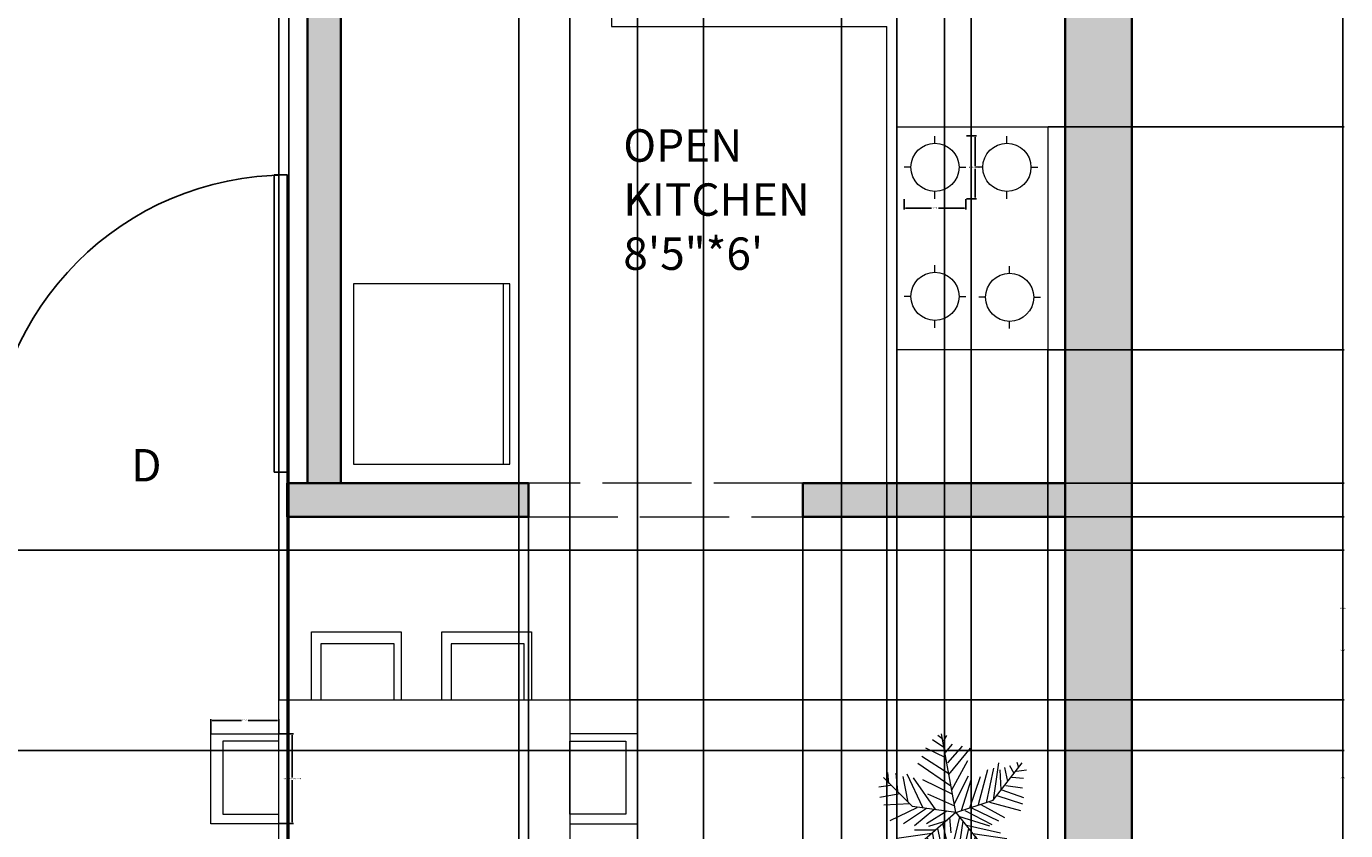
# Model space of a CAD drawing. Units: inches. Extents: x 2035 to 2384, y 1427 to 2020.
# Tile 6 of 7: x 2206 to 2384, y 1794 to 1902. Entities that reach past the tile are written whole.
import ezdxf

# ---------------------------------------------------------------- set-up
doc = ezdxf.new("R2010")
doc.units = ezdxf.units.IN
doc.linetypes.add('ACAD_ISO02W100', pattern=[15, 12, -3])
for name, color, linetype, lineweight in [('A-ANNO-DIMS', 2, 'Continuous', 18), ('A-ANNO-IDEN', 201, 'Continuous', 18), ('A-AREA-IDEN', 201, 'Continuous', 18), ('A-EQPM', 71, 'Continuous', 18), ('A-FLOR-CABN', 71, 'Continuous', 18), ('A-WALL-OVHD', 140, 'ACAD_ISO02W100', 18), ('A-WALL-PATT', 140, 'Continuous', 13), ('C-PROP', 7, 'Continuous', 25), ('DOOR', 52, 'Continuous', 25), ('FUR', 71, 'Continuous', 18), ('L-PLNT', 112, 'Continuous', 18), ('WALL', 140, 'Continuous', 35)]:
    doc.layers.add(name, color=color, linetype=linetype, lineweight=lineweight)
doc.styles.get("Standard").update_dxf_attribs({"font": 'arial.ttf'})
doc.dimstyles.get("Standard").update_dxf_attribs({"dimtxt": 0.18, "dimasz": 0.18, "dimexe": 0.18, "dimexo": 0.0625, "dimgap": 0.09, "dimtad": 0, "dimtih": 1, "dimtoh": 1, "dimdec": 4, "dimzin": 0, "dimdsep": 46, "dimtxsty": 'Standard', "dimcen": 0.09, "dimadec": 0, "dimazin": 0, "dimtfac": 1, "dimtdec": 4, "dimtofl": 0, "dimtmove": 0, "dimatfit": 3, "dimfxl": 1, "dimtolj": 1, "dimtzin": 0, "dimarcsym": 0})

# ---------------------------------------------------------------- blocks, each defined once
blk = doc.blocks.new('*U2')
for p, q in [((0, 0), (0, -6)), ((40, 0), (40, -6))]:
    blk.add_line(p, q)
blk.add_lwpolyline([(0, 0), (0, 40), (1.75, 40), (1.75, 0)], close=True)
blk.add_arc((0, 0), 40, 0, 90)
blk = doc.blocks.new('*U6')
for p, q in [((-8.737, 47.138), (-17.069, 52.711)), ((-10.186, 53.64), (-13.084, 55.962)), ((0, 0), (-10.5, 57)), ((-9.099, 51.782), (-6.563, 55.962)), ((-7.65, 43.423), (-2.578, 49.46)), ((-5.839, 35.992), (4.667, 48.067)), ((-5.114, 28.097), (-24.676, 40.636)), ((-7.288, 39.707), (-21.778, 46.673)), ((-5.114, 27.632), (10.463, 46.673)), ((-48.585, 21.131), (-49.309, 29.026)), ((-3.665, 19.273), (-27.574, 35.527)), ((-2.941, 16.486), (8.652, 37.85)), ((16.259, 5.805), (23.142, 31.348)), ((22.055, 7.198), (27.489, 32.277)), ((27, 9), (48, 36)), ((27.127, 9.056), (31.112, 35.992)), ((31.836, 30.883), (32.561, 16.486)), ((35.096, 32.741), (37.27, 22.524)), ((38.719, 34.134), (41.979, 28.561)), ((43.791, 29.954), (51.036, 30.883)), ((44.153, 36.456), (45.239, 32.741)), ((-47.498, 19.737), (-55.83, 18.344)), ((-31.5, 4.5), (-52.5, 25.5)), ((-43.513, 28.561), (-42.427, 15.558)), ((-38.442, 26.239), (-34.819, 7.663)), ((-35.544, 28.097), (-24.314, 3.947)), ((-14.533, 2.09), (-30.834, 25.31)), ((-24.314, 23.917), (-2.941, 13.7)), ((-1.129, 6.734), (9.014, 26.704)), ((3.942, 1.625), (11.187, 24.381)), ((10.101, 3.483), (17.708, 26.239)), ((36.183, 19.737), (48.137, 17.88)), ((40.53, 25.775), (48.862, 24.846)), ((-40.615, 13.7), (-55.105, 10.913)), ((-20.691, 13.7), (-1.129, 4.876)), ((29.662, 12.307), (48.137, 6.269)), ((33.285, 16.486), (48.862, 10.913)), ((-33.37, 6.269), (-52.207, 5.34)), ((-28.299, 3.483), (-47.86, -5.805)), ((-21.416, 3.018), (-38.079, -8.128)), ((0, 0), (-31.5, 4.5)), ((-15.982, 2.09), (-30.11, -9.521)), ((0, 0), (-22.5, -19.5)), ((-6.563, 1.161), (-21.416, -8.128)), ((0, 0), (27, 9)), ((0, 0), (18, -22.5)), ((6.478, 1.625), (26.04, -8.592)), ((11.187, 3.483), (30.749, -5.805)), ((18.07, 5.805), (35.096, -3.483)), ((24.229, 7.663), (46.688, 1.625)), ((-6.563, -5.805), (-19.967, -9.985)), ((-9.461, -8.592), (-6.201, -23.453)), ((-4.752, -3.483), (-3.665, -14.629)), ((2.493, -3.019), (-1.491, -20.202)), ((1.769, -2.555), (24.229, -9.521)), ((5.029, -6.27), (2.131, -25.775)), ((7.565, -9.056), (32.198, -14.629)), ((-17.431, -15.094), (-42.789, -18.809)), ((-15.257, -12.772), (-30.11, -12.772)), ((-20.691, -18.345), (-17.793, -44.352)), ((-17.069, -15.094), (-12.721, -40.172)), ((-13.446, -11.378), (-8.737, -32.741)), ((9.014, -11.378), (3.58, -35.992)), ((14.085, -16.951), (6.478, -40.172)), ((12.274, -15.094), (36.907, -18.809)), ((-24.314, -21.596), (-42.427, -22.06)), ((-26.849, -26.24), (-40.253, -25.775)), ((-22.5, -19.5), (-37.5, -45)), ((-25.038, -23.918), (-22.865, -45.281)), ((18.07, -22.524), (8.289, -45.745)), ((16.259, -19.738), (36.183, -22.989)), ((18, -22.5), (27, -52.5)), ((18.433, -22.524), (40.53, -29.026)), ((19.157, -25.311), (38.719, -33.206)), ((-28.299, -29.026), (-42.789, -31.348)), ((-30.834, -34.135), (-42.427, -35.528)), ((-32.646, -36.921), (-31.921, -44.352)), ((-29.023, -30.884), (-27.936, -43.887)), ((20.244, -30.419), (15.897, -44.816)), ((22.78, -37.85), (19.519, -48.532)), ((21.331, -32.741), (39.081, -40.636)), ((-34.457, -39.708), (-40.978, -42.494)), ((22.78, -38.314), (34.372, -44.816)), ((24.591, -45.745), (23.142, -50.854)), ((24.591, -43.423), (30.749, -47.603)), ((26.764, -49.925), (28.213, -50.854))]:
    blk.add_line(p, q)
blk = doc.blocks.new('CHAIR-DINING')
for p, q in [((0, 0), (0, 9.14)), ((0, 9.14), (12.09, 9.14)), ((12.09, 9.14), (12.09, 0))]:
    blk.add_line(p, q)
blk.add_lwpolyline([(1.26, 0), (11.11, 0), (11.11, 7.54), (1.26, 7.54)], close=True)
blk = doc.blocks.new('COOKTOP-BURNER')
for p, q in [((4.16, 7.46), (4.16, 8.43)), ((0.92, 4.22), (0, 4.22)), ((7.4, 4.22), (8.32, 4.22)), ((4.16, 0), (4.16, 0.98))]:
    blk.add_line(p, q)
blk.add_circle((4.16, 4.22), 3.24)
blk = doc.blocks.new('*D16')
at = {"layer": 'A-ANNO-DIMS', "color": 0, "lineweight": -2, "transparency": 16777216}
for p, q in [((2239.94, 1806.65), (2241.87, 1806.65)), ((2241.69, 1806.47), (2241.69, 1800.79)), ((2241.69, 1794.75), (2241.69, 1800.43)), ((2239.94, 1794.57), (2241.87, 1794.57))]:
    blk.add_line(p, q, dxfattribs=at)
at = {"layer": 'A-ANNO-DIMS', "color": 0, "lineweight": 100, "transparency": 16777216}
for points in [[(2241.66, 1806.47), (2241.72, 1806.47), (2241.69, 1806.65)], [(2241.66, 1794.75), (2241.72, 1794.75), (2241.69, 1794.57)]]:
    blk.add_solid(points, dxfattribs=at)
at = {"layer": 'Defpoints', "color": 0, "lineweight": 100, "transparency": 16777216}
for p in [(2239.88, 1806.65), (2241.69, 1806.65), (2239.88, 1794.57)]:
    blk.add_point(p, dxfattribs=at)
at = {"layer": 'A-ANNO-DIMS', "color": 0, "transparency": 16777216, "insert": (2241.69, 1800.61), "char_height": 0.18, "attachment_point": 5}
blk.add_mtext('\\A1;DINING CHAIR 12 TYP.', dxfattribs=at)
blk = doc.blocks.new('*D17')
at = {"layer": 'A-ANNO-DIMS', "color": 0, "lineweight": -2, "transparency": 16777216}
for p, q in [((2230.74, 1806.72), (2230.74, 1808.65)), ((2230.92, 1808.47), (2234.85, 1808.47)), ((2239.7, 1808.47), (2235.77, 1808.47)), ((2239.88, 1806.72), (2239.88, 1808.65))]:
    blk.add_line(p, q, dxfattribs=at)
at = {"layer": 'A-ANNO-DIMS', "color": 0, "lineweight": 100, "transparency": 16777216}
for points in [[(2230.92, 1808.5), (2230.92, 1808.44), (2230.74, 1808.47)], [(2239.7, 1808.5), (2239.7, 1808.44), (2239.88, 1808.47)]]:
    blk.add_solid(points, dxfattribs=at)
at = {"layer": 'Defpoints', "color": 0, "lineweight": 100, "transparency": 16777216}
for p in [(2230.74, 1808.47), (2230.74, 1806.65), (2239.88, 1806.65)]:
    blk.add_point(p, dxfattribs=at)
at = {"layer": 'A-ANNO-DIMS', "color": 0, "transparency": 16777216, "insert": (2235.31, 1808.47), "char_height": 0.18, "attachment_point": 5}
blk.add_mtext('\\A1;9 TYP.', dxfattribs=at)
blk = doc.blocks.new('*D20')
at = {"layer": 'A-ANNO-DIMS', "color": 0, "lineweight": -2, "transparency": 16777216}
for p, q in [((2332.46, 1887.13), (2333.84, 1887.13)), ((2333.66, 1886.95), (2333.66, 1883.09)), ((2333.66, 1878.87), (2333.66, 1882.73)), ((2332.46, 1878.69), (2333.84, 1878.69))]:
    blk.add_line(p, q, dxfattribs=at)
at = {"layer": 'A-ANNO-DIMS', "color": 0, "lineweight": 100, "transparency": 16777216}
for points in [[(2333.63, 1886.95), (2333.69, 1886.95), (2333.66, 1887.13)], [(2333.63, 1878.87), (2333.69, 1878.87), (2333.66, 1878.69)]]:
    blk.add_solid(points, dxfattribs=at)
at = {"layer": 'Defpoints', "color": 0, "lineweight": 100, "transparency": 16777216}
for p in [(2332.39, 1887.13), (2333.66, 1887.13), (2332.39, 1878.69)]:
    blk.add_point(p, dxfattribs=at)
at = {"layer": 'A-ANNO-DIMS', "color": 0, "transparency": 16777216, "insert": (2333.66, 1882.91), "char_height": 0.18, "attachment_point": 5}
blk.add_mtext('\\A1;BURNER 8 TYP.', dxfattribs=at)
blk = doc.blocks.new('*D21')
at = {"layer": 'A-ANNO-DIMS', "color": 0, "lineweight": -2, "transparency": 16777216}
for p, q in [((2324.08, 1878.63), (2324.08, 1877.25)), ((2332.39, 1878.63), (2332.39, 1877.25)), ((2324.26, 1877.43), (2327.78, 1877.43)), ((2332.21, 1877.43), (2328.69, 1877.43))]:
    blk.add_line(p, q, dxfattribs=at)
at = {"layer": 'A-ANNO-DIMS', "color": 0, "lineweight": 100, "transparency": 16777216}
for points in [[(2324.26, 1877.46), (2324.26, 1877.4), (2324.08, 1877.43)], [(2332.21, 1877.46), (2332.21, 1877.4), (2332.39, 1877.43)]]:
    blk.add_solid(points, dxfattribs=at)
at = {"layer": 'Defpoints', "color": 0, "lineweight": 100, "transparency": 16777216}
for p in [(2324.08, 1878.69), (2332.39, 1878.69), (2332.39, 1877.43)]:
    blk.add_point(p, dxfattribs=at)
at = {"layer": 'A-ANNO-DIMS', "color": 0, "transparency": 16777216, "insert": (2328.23, 1877.43), "char_height": 0.18, "attachment_point": 5}
blk.add_mtext('\\A1;8 TYP.', dxfattribs=at)
blk = doc.blocks.new('*D23')
at = {"layer": 'A-ANNO-DIMS', "color": 0, "lineweight": -2, "transparency": 16777216}
for p, q in [((2354.82, 1981.38), (2383.33, 1981.38)), ((2383.15, 1981.2), (2383.15, 1741.56)), ((2383.15, 1501.56), (2383.15, 1741.2)), ((2354.82, 1501.38), (2383.33, 1501.38))]:
    blk.add_line(p, q, dxfattribs=at)
at = {"layer": 'A-ANNO-DIMS', "color": 0, "lineweight": 100, "transparency": 16777216}
for points in [[(2383.12, 1981.2), (2383.18, 1981.2), (2383.15, 1981.38)], [(2383.12, 1501.56), (2383.18, 1501.56), (2383.15, 1501.38)]]:
    blk.add_solid(points, dxfattribs=at)
at = {"layer": 'Defpoints', "color": 0, "lineweight": 100, "transparency": 16777216}
for p in [(2354.75, 1981.38), (2383.15, 1981.38), (2354.75, 1501.38)]:
    blk.add_point(p, dxfattribs=at)
at = {"layer": 'A-ANNO-DIMS', "color": 0, "transparency": 16777216, "insert": (2383.15, 1741.38), "char_height": 0.18, "attachment_point": 5}
blk.add_mtext('\\A1;480', dxfattribs=at)
blk = doc.blocks.new('*D25')
at = {"layer": 'A-ANNO-DIMS', "color": 0, "lineweight": -2, "transparency": 16777216}
for p, q in [((2241.25, 1503.69), (2241.25, 2009.96)), ((2241.43, 2009.78), (2256.26, 2009.78)), ((2272.01, 2009.78), (2257.18, 2009.78)), ((2272.19, 1503.69), (2272.19, 2009.96))]:
    blk.add_line(p, q, dxfattribs=at)
at = {"layer": 'A-ANNO-DIMS', "color": 0, "lineweight": 100, "transparency": 16777216}
for points in [[(2241.43, 2009.81), (2241.43, 2009.75), (2241.25, 2009.78)], [(2272.01, 2009.81), (2272.01, 2009.75), (2272.19, 2009.78)]]:
    blk.add_solid(points, dxfattribs=at)
at = {"layer": 'Defpoints', "color": 0, "lineweight": 100, "transparency": 16777216}
for p in [(2272.19, 2009.78), (2241.25, 1503.63), (2272.19, 1503.63)]:
    blk.add_point(p, dxfattribs=at)
at = {"layer": 'A-ANNO-DIMS', "color": 0, "transparency": 16777216, "insert": (2256.72, 2009.78), "char_height": 0.18, "attachment_point": 5}
blk.add_mtext('\\A1;30.935', dxfattribs=at)
blk = doc.blocks.new('*D26')
at = {"layer": 'A-ANNO-DIMS', "color": 0, "lineweight": -2, "transparency": 16777216}
for p, q in [((2272.19, 1506.56), (2272.19, 2009.96)), ((2272.37, 2009.78), (2297.26, 2009.78)), ((2322.93, 2009.78), (2298.04, 2009.78)), ((2323.11, 1506.56), (2323.11, 2009.96))]:
    blk.add_line(p, q, dxfattribs=at)
at = {"layer": 'A-ANNO-DIMS', "color": 0, "lineweight": 100, "transparency": 16777216}
for points in [[(2272.37, 2009.81), (2272.37, 2009.75), (2272.19, 2009.78)], [(2322.93, 2009.81), (2322.93, 2009.75), (2323.11, 2009.78)]]:
    blk.add_solid(points, dxfattribs=at)
at = {"layer": 'Defpoints', "color": 0, "lineweight": 100, "transparency": 16777216}
for p in [(2323.11, 2009.78), (2272.19, 1506.5), (2323.11, 1506.5)]:
    blk.add_point(p, dxfattribs=at)
at = {"layer": 'A-ANNO-DIMS', "color": 0, "transparency": 16777216, "insert": (2297.65, 2009.78), "char_height": 0.18, "attachment_point": 5}
blk.add_mtext('\\A1;50.92', dxfattribs=at)
blk = doc.blocks.new('*D38')
at = {"layer": 'A-ANNO-DIMS', "color": 0, "lineweight": -2, "transparency": 16777216}
for p, q in [((2183.82, 1831.37), (2383.33, 1831.37)), ((2383.15, 1831.19), (2383.15, 1818.07)), ((2383.15, 1804.58), (2383.15, 1817.7)), ((2183.82, 1804.4), (2383.33, 1804.4))]:
    blk.add_line(p, q, dxfattribs=at)
at = {"layer": 'A-ANNO-DIMS', "color": 0, "lineweight": 100, "transparency": 16777216}
for points in [[(2383.12, 1831.19), (2383.18, 1831.19), (2383.15, 1831.37)], [(2383.12, 1804.58), (2383.18, 1804.58), (2383.15, 1804.4)]]:
    blk.add_solid(points, dxfattribs=at)
at = {"layer": 'Defpoints', "color": 0, "lineweight": 100, "transparency": 16777216}
for p in [(2183.75, 1831.37), (2383.15, 1831.37), (2183.75, 1804.4)]:
    blk.add_point(p, dxfattribs=at)
at = {"layer": 'A-ANNO-DIMS', "color": 0, "transparency": 16777216, "insert": (2383.15, 1817.88), "char_height": 0.18, "attachment_point": 5}
blk.add_mtext('\\A1;26.97', dxfattribs=at)
blk = doc.blocks.new('*D40')
at = {"layer": 'A-ANNO-DIMS', "color": 0, "lineweight": -2, "transparency": 16777216}
for p, q in [((2201.01, 1835.82), (2201.01, 1427.17)), ((2241.01, 1835.82), (2241.01, 1427.17)), ((2201.19, 1427.35), (2220.79, 1427.35)), ((2240.83, 1427.35), (2221.24, 1427.35))]:
    blk.add_line(p, q, dxfattribs=at)
at = {"layer": 'A-ANNO-DIMS', "color": 0, "lineweight": 100, "transparency": 16777216}
for points in [[(2201.19, 1427.38), (2201.19, 1427.32), (2201.01, 1427.35)], [(2240.83, 1427.38), (2240.83, 1427.32), (2241.01, 1427.35)]]:
    blk.add_solid(points, dxfattribs=at)
at = {"layer": 'Defpoints', "color": 0, "lineweight": 100, "transparency": 16777216}
for p in [(2201.01, 1835.88), (2241.01, 1835.88), (2241.01, 1427.35)]:
    blk.add_point(p, dxfattribs=at)
at = {"layer": 'A-ANNO-DIMS', "color": 0, "transparency": 16777216, "insert": (2221.01, 1427.35), "char_height": 0.18, "attachment_point": 5}
blk.add_mtext('\\A1;40', dxfattribs=at)
blk = doc.blocks.new('*D41')
at = {"layer": 'A-ANNO-DIMS', "color": 0, "lineweight": -2, "transparency": 16777216}
for p, q in [((2273.51, 1840.32), (2273.51, 1427.17)), ((2310.46, 1840.32), (2310.46, 1427.17)), ((2273.69, 1427.35), (2291.59, 1427.35)), ((2310.28, 1427.35), (2292.38, 1427.35))]:
    blk.add_line(p, q, dxfattribs=at)
at = {"layer": 'A-ANNO-DIMS', "color": 0, "lineweight": 100, "transparency": 16777216}
for points in [[(2273.69, 1427.38), (2273.69, 1427.32), (2273.51, 1427.35)], [(2310.28, 1427.38), (2310.28, 1427.32), (2310.46, 1427.35)]]:
    blk.add_solid(points, dxfattribs=at)
at = {"layer": 'Defpoints', "color": 0, "lineweight": 100, "transparency": 16777216}
for p in [(2273.51, 1840.38), (2310.46, 1840.38), (2310.46, 1427.35)]:
    blk.add_point(p, dxfattribs=at)
at = {"layer": 'A-ANNO-DIMS', "color": 0, "transparency": 16777216, "insert": (2291.98, 1427.35), "char_height": 0.18, "attachment_point": 5}
blk.add_mtext('\\A1;36.95', dxfattribs=at)
blk = doc.blocks.new('*D42')
at = {"layer": 'A-ANNO-DIMS', "color": 0, "lineweight": -2, "transparency": 16777216}
for p, q in [((2297.05, 1925.82), (2297.05, 1427.17)), ((2333.11, 1925.82), (2333.11, 1427.17)), ((2297.23, 1427.35), (2314.69, 1427.35)), ((2332.93, 1427.35), (2315.47, 1427.35))]:
    blk.add_line(p, q, dxfattribs=at)
at = {"layer": 'A-ANNO-DIMS', "color": 0, "lineweight": 100, "transparency": 16777216}
for points in [[(2297.23, 1427.38), (2297.23, 1427.32), (2297.05, 1427.35)], [(2332.93, 1427.38), (2332.93, 1427.32), (2333.11, 1427.35)]]:
    blk.add_solid(points, dxfattribs=at)
at = {"layer": 'Defpoints', "color": 0, "lineweight": 100, "transparency": 16777216}
for p in [(2297.05, 1925.88), (2333.11, 1925.88), (2333.11, 1427.35)]:
    blk.add_point(p, dxfattribs=at)
at = {"layer": 'A-ANNO-DIMS', "color": 0, "transparency": 16777216, "insert": (2315.08, 1427.35), "char_height": 0.18, "attachment_point": 5}
blk.add_mtext('\\A1;36.06', dxfattribs=at)
blk = doc.blocks.new('*D45')
at = {"layer": 'A-ANNO-DIMS', "color": 0, "lineweight": -2, "transparency": 16777216}
for p, q in [((2321.75, 1840.32), (2321.75, 1427.17)), ((2345.75, 1840.32), (2345.75, 1427.17)), ((2321.93, 1427.35), (2333.53, 1427.35)), ((2345.57, 1427.35), (2333.97, 1427.35))]:
    blk.add_line(p, q, dxfattribs=at)
at = {"layer": 'A-ANNO-DIMS', "color": 0, "lineweight": 100, "transparency": 16777216}
for points in [[(2321.93, 1427.38), (2321.93, 1427.32), (2321.75, 1427.35)], [(2345.57, 1427.38), (2345.57, 1427.32), (2345.75, 1427.35)]]:
    blk.add_solid(points, dxfattribs=at)
at = {"layer": 'Defpoints', "color": 0, "lineweight": 100, "transparency": 16777216}
for p in [(2321.75, 1840.38), (2345.75, 1840.38), (2345.75, 1427.35)]:
    blk.add_point(p, dxfattribs=at)
at = {"layer": 'A-ANNO-DIMS', "color": 0, "transparency": 16777216, "insert": (2333.75, 1427.35), "char_height": 0.18, "attachment_point": 5}
blk.add_mtext('\\A1;24', dxfattribs=at)
blk = doc.blocks.new('*D46')
at = {"layer": 'A-ANNO-DIMS', "color": 0, "lineweight": -2, "transparency": 16777216}
for p, q in [((2288.19, 1905.68), (2288.19, 1427.17)), ((2315.66, 1905.68), (2315.66, 1427.17)), ((2288.37, 1427.35), (2301.53, 1427.35)), ((2315.48, 1427.35), (2302.32, 1427.35))]:
    blk.add_line(p, q, dxfattribs=at)
at = {"layer": 'A-ANNO-DIMS', "color": 0, "lineweight": 100, "transparency": 16777216}
for points in [[(2288.37, 1427.38), (2288.37, 1427.32), (2288.19, 1427.35)], [(2315.48, 1427.38), (2315.48, 1427.32), (2315.66, 1427.35)]]:
    blk.add_solid(points, dxfattribs=at)
at = {"layer": 'Defpoints', "color": 0, "lineweight": 100, "transparency": 16777216}
for p in [(2288.19, 1905.75), (2315.66, 1905.75), (2315.66, 1427.35)]:
    blk.add_point(p, dxfattribs=at)
at = {"layer": 'A-ANNO-DIMS', "color": 0, "transparency": 16777216, "insert": (2301.92, 1427.35), "char_height": 0.18, "attachment_point": 5}
blk.add_mtext('\\A1;27.47', dxfattribs=at)
blk = doc.blocks.new('*D48')
at = {"layer": 'A-ANNO-DIMS', "color": 0, "lineweight": -2, "transparency": 16777216}
for p, q in [((2323.12, 1858.3), (2323.12, 1427.17)), ((2343.42, 1858.3), (2343.42, 1427.17)), ((2323.3, 1427.35), (2332.81, 1427.35)), ((2343.24, 1427.35), (2333.74, 1427.35))]:
    blk.add_line(p, q, dxfattribs=at)
at = {"layer": 'A-ANNO-DIMS', "color": 0, "lineweight": 100, "transparency": 16777216}
for points in [[(2323.3, 1427.38), (2323.3, 1427.32), (2323.12, 1427.35)], [(2343.24, 1427.38), (2343.24, 1427.32), (2343.42, 1427.35)]]:
    blk.add_solid(points, dxfattribs=at)
at = {"layer": 'Defpoints', "color": 0, "lineweight": 100, "transparency": 16777216}
for p in [(2323.12, 1858.36), (2343.42, 1858.36), (2343.42, 1427.35)]:
    blk.add_point(p, dxfattribs=at)
at = {"layer": 'A-ANNO-DIMS', "color": 0, "transparency": 16777216, "insert": (2333.27, 1427.35), "char_height": 0.18, "attachment_point": 5}
blk.add_mtext('\\A1;20.302', dxfattribs=at)
blk = doc.blocks.new('*D49')
at = {"layer": 'A-ANNO-DIMS', "color": 0, "lineweight": -2, "transparency": 16777216}
for p, q in [((2343.49, 1888.36), (2383.33, 1888.36)), ((2383.15, 1888.18), (2383.15, 1873.54)), ((2383.15, 1858.54), (2383.15, 1873.18)), ((2343.49, 1858.36), (2383.33, 1858.36))]:
    blk.add_line(p, q, dxfattribs=at)
at = {"layer": 'A-ANNO-DIMS', "color": 0, "lineweight": 100, "transparency": 16777216}
for points in [[(2383.12, 1888.18), (2383.18, 1888.18), (2383.15, 1888.36)], [(2383.12, 1858.54), (2383.18, 1858.54), (2383.15, 1858.36)]]:
    blk.add_solid(points, dxfattribs=at)
at = {"layer": 'Defpoints', "color": 0, "lineweight": 100, "transparency": 16777216}
for p in [(2343.42, 1888.36), (2383.15, 1888.36), (2343.42, 1858.36)]:
    blk.add_point(p, dxfattribs=at)
at = {"layer": 'A-ANNO-DIMS', "color": 0, "transparency": 16777216, "insert": (2383.15, 1873.36), "char_height": 0.18, "attachment_point": 5}
blk.add_mtext('\\A1;30', dxfattribs=at)
blk = doc.blocks.new('*D54')
at = {"layer": 'A-ANNO-DIMS', "color": 0, "lineweight": -2, "transparency": 16777216}
for p, q in [((2239.88, 1811.3), (2239.88, 2009.96)), ((2240.06, 2009.78), (2259.08, 2009.78)), ((2278.89, 2009.78), (2259.87, 2009.78)), ((2279.07, 1811.3), (2279.07, 2009.96))]:
    blk.add_line(p, q, dxfattribs=at)
at = {"layer": 'A-ANNO-DIMS', "color": 0, "lineweight": 100, "transparency": 16777216}
for points in [[(2240.06, 2009.81), (2240.06, 2009.75), (2239.88, 2009.78)], [(2278.89, 2009.81), (2278.89, 2009.75), (2279.07, 2009.78)]]:
    blk.add_solid(points, dxfattribs=at)
at = {"layer": 'Defpoints', "color": 0, "lineweight": 100, "transparency": 16777216}
for p in [(2279.07, 2009.78), (2239.88, 1811.24), (2279.07, 1811.24)]:
    blk.add_point(p, dxfattribs=at)
at = {"layer": 'A-ANNO-DIMS', "color": 0, "transparency": 16777216, "insert": (2259.47, 2009.78), "char_height": 0.18, "attachment_point": 5}
blk.add_mtext('\\A1;39.19', dxfattribs=at)
blk = doc.blocks.new('*D55')
at = {"layer": 'A-ANNO-DIMS', "color": 0, "lineweight": -2, "transparency": 16777216}
for p, q in [((2279.13, 1811.24), (2383.33, 1811.24)), ((2383.15, 1811.06), (2383.15, 1800.94)), ((2383.15, 1790.46), (2383.15, 1800.57)), ((2279.13, 1790.28), (2383.33, 1790.28))]:
    blk.add_line(p, q, dxfattribs=at)
at = {"layer": 'A-ANNO-DIMS', "color": 0, "lineweight": 100, "transparency": 16777216}
for points in [[(2383.12, 1811.06), (2383.18, 1811.06), (2383.15, 1811.24)], [(2383.12, 1790.46), (2383.18, 1790.46), (2383.15, 1790.28)]]:
    blk.add_solid(points, dxfattribs=at)
at = {"layer": 'Defpoints', "color": 0, "lineweight": 100, "transparency": 16777216}
for p in [(2279.07, 1811.24), (2383.15, 1811.24), (2279.07, 1790.28)]:
    blk.add_point(p, dxfattribs=at)
at = {"layer": 'A-ANNO-DIMS', "color": 0, "transparency": 16777216, "insert": (2383.15, 1800.76), "char_height": 0.18, "attachment_point": 5}
blk.add_mtext('\\A1;20.96', dxfattribs=at)
blk = doc.blocks.new('*D59')
at = {"layer": 'A-ANNO-DIMS', "color": 0, "lineweight": -2, "transparency": 16777216}
for p, q in [((2354.82, 1981.38), (2383.33, 1981.38)), ((2383.15, 1981.2), (2383.15, 1911.06)), ((2383.15, 1840.56), (2383.15, 1910.7)), ((2345.82, 1840.38), (2383.33, 1840.38))]:
    blk.add_line(p, q, dxfattribs=at)
at = {"layer": 'A-ANNO-DIMS', "color": 0, "lineweight": 100, "transparency": 16777216}
for points in [[(2383.12, 1981.2), (2383.18, 1981.2), (2383.15, 1981.38)], [(2383.12, 1840.56), (2383.18, 1840.56), (2383.15, 1840.38)]]:
    blk.add_solid(points, dxfattribs=at)
at = {"layer": 'Defpoints', "color": 0, "lineweight": 100, "transparency": 16777216}
for p in [(2354.75, 1981.38), (2383.15, 1981.38), (2345.75, 1840.38)]:
    blk.add_point(p, dxfattribs=at)
at = {"layer": 'A-ANNO-DIMS', "color": 0, "transparency": 16777216, "insert": (2383.15, 1910.88), "char_height": 0.18, "attachment_point": 5}
blk.add_mtext('\\A1;141', dxfattribs=at)
blk = doc.blocks.new('*D60')
at = {"layer": 'A-ANNO-DIMS', "color": 0, "lineweight": -2, "transparency": 16777216}
for p, q in [((2193.76, 1860.83), (2193.76, 2009.96)), ((2193.94, 2009.78), (2218.54, 2009.78)), ((2243.57, 2009.78), (2218.97, 2009.78)), ((2243.75, 1840.44), (2243.75, 2009.96))]:
    blk.add_line(p, q, dxfattribs=at)
at = {"layer": 'A-ANNO-DIMS', "color": 0, "lineweight": 100, "transparency": 16777216}
for points in [[(2193.94, 2009.81), (2193.94, 2009.75), (2193.76, 2009.78)], [(2243.57, 2009.81), (2243.57, 2009.75), (2243.75, 2009.78)]]:
    blk.add_solid(points, dxfattribs=at)
at = {"layer": 'Defpoints', "color": 0, "lineweight": 100, "transparency": 16777216}
for p in [(2243.75, 2009.78), (2193.76, 1860.77), (2243.75, 1840.38)]:
    blk.add_point(p, dxfattribs=at)
at = {"layer": 'A-ANNO-DIMS', "color": 0, "transparency": 16777216, "insert": (2218.75, 2009.78), "char_height": 0.18, "attachment_point": 5}
blk.add_mtext('\\A1;50', dxfattribs=at)
blk = doc.blocks.new('*D66')
at = {"layer": 'A-ANNO-DIMS', "color": 0, "lineweight": -2, "transparency": 16777216}
for p, q in [((2345.82, 1835.88), (2383.33, 1835.88)), ((2383.15, 1835.7), (2383.15, 1823.74)), ((2383.15, 1811.42), (2383.15, 1823.38)), ((2279.13, 1811.24), (2383.33, 1811.24))]:
    blk.add_line(p, q, dxfattribs=at)
at = {"layer": 'A-ANNO-DIMS', "color": 0, "lineweight": 100, "transparency": 16777216}
for points in [[(2383.12, 1835.7), (2383.18, 1835.7), (2383.15, 1835.88)], [(2383.12, 1811.42), (2383.18, 1811.42), (2383.15, 1811.24)]]:
    blk.add_solid(points, dxfattribs=at)
at = {"layer": 'Defpoints', "color": 0, "lineweight": 100, "transparency": 16777216}
for p in [(2345.75, 1835.88), (2383.15, 1835.88), (2279.07, 1811.24)]:
    blk.add_point(p, dxfattribs=at)
at = {"layer": 'A-ANNO-DIMS', "color": 0, "transparency": 16777216, "insert": (2383.15, 1823.56), "char_height": 0.18, "attachment_point": 5}
blk.add_mtext('\\A1;24.646', dxfattribs=at)
blk = doc.blocks.new('*D68')
at = {"layer": 'A-ANNO-DIMS', "color": 0, "lineweight": -2, "transparency": 16777216}
for p, q in [((2329.51, 1685.44), (2329.51, 2009.96)), ((2329.69, 2009.78), (2337.25, 2009.78)), ((2345.57, 2009.78), (2338.02, 2009.78)), ((2345.75, 1685.44), (2345.75, 2009.96))]:
    blk.add_line(p, q, dxfattribs=at)
at = {"layer": 'A-ANNO-DIMS', "color": 0, "lineweight": 100, "transparency": 16777216}
for points in [[(2329.69, 2009.81), (2329.69, 2009.75), (2329.51, 2009.78)], [(2345.57, 2009.81), (2345.57, 2009.75), (2345.75, 2009.78)]]:
    blk.add_solid(points, dxfattribs=at)
at = {"layer": 'Defpoints', "color": 0, "lineweight": 100, "transparency": 16777216}
for p in [(2345.75, 2009.78), (2329.51, 1685.38), (2345.75, 1685.38)]:
    blk.add_point(p, dxfattribs=at)
at = {"layer": 'A-ANNO-DIMS', "color": 0, "transparency": 16777216, "insert": (2337.63, 2009.78), "char_height": 0.18, "attachment_point": 5}
blk.add_mtext('\\A1;16.24', dxfattribs=at)
blk = doc.blocks.new('*D70')
at = {"layer": 'A-ANNO-DIMS', "color": 0, "lineweight": -2, "transparency": 16777216}
for p, q in [((2188.25, 1804.46), (2188.25, 2009.96)), ((2188.43, 2009.78), (2213.67, 2009.78)), ((2239.7, 2009.78), (2214.46, 2009.78)), ((2239.88, 1811.3), (2239.88, 2009.96))]:
    blk.add_line(p, q, dxfattribs=at)
at = {"layer": 'A-ANNO-DIMS', "color": 0, "lineweight": 100, "transparency": 16777216}
for points in [[(2188.43, 2009.81), (2188.43, 2009.75), (2188.25, 2009.78)], [(2239.7, 2009.81), (2239.7, 2009.75), (2239.88, 2009.78)]]:
    blk.add_solid(points, dxfattribs=at)
at = {"layer": 'Defpoints', "color": 0, "lineweight": 100, "transparency": 16777216}
for p in [(2239.88, 2009.78), (2239.88, 1811.24), (2188.25, 1804.39)]:
    blk.add_point(p, dxfattribs=at)
at = {"layer": 'A-ANNO-DIMS', "color": 0, "transparency": 16777216, "insert": (2214.07, 2009.78), "char_height": 0.18, "attachment_point": 5}
blk.add_mtext('\\A1;51.62', dxfattribs=at)

msp = doc.modelspace()

# ---------------------------------------------------------------- hatches: boundary and pattern name
at = {"layer": 'A-WALL-PATT'}
h = msp.add_hatch(color=256, dxfattribs=at)
h.dxf.hatch_style = 1
h.paths.add_polyline_path([(2145.6215, 1981.3816), (2123.7529, 1981.3816), (2123.7529, 1972.3816), (2145.6215, 1972.3816)])
h.paths.add_polyline_path([(2354.7529, 1981.3816), (2209.3767, 1981.3816), (2209.3767, 1972.3816), (2354.7529, 1972.3816)])
h.paths.add_polyline_path([(2123.7529, 1981.3816), (2114.7529, 1981.3816), (2114.7529, 1505.8816), (2123.7529, 1505.8816)])
h.paths.add_polyline_path([(2248.2529, 1928.1316), (2243.7529, 1928.1316), (2243.7529, 1840.3816), (2248.2529, 1840.3816)])
h.paths.add_polyline_path([(2297.0514, 1930.3816), (2284.6994, 1930.3816), (2284.6994, 1925.8816), (2297.0514, 1925.8816)])
h.paths.add_polyline_path([(2345.7529, 1930.3816), (2333.1098, 1930.3816), (2333.1098, 1925.8816), (2345.7529, 1925.8816)])
h.paths.add_polyline_path([(2354.7529, 1972.3816), (2345.7529, 1972.3816), (2345.7529, 1501.3816), (2354.7529, 1501.3816)])
h.paths.add_polyline_path([(2188.2529, 1835.8816), (2183.7529, 1835.8816), (2183.7529, 1831.3677), (2184.207, 1831.3677), (2188.2529, 1831.3677)])
h.paths.add_polyline_path([(2188.2529, 1804.3949), (2184.207, 1804.3949), (2183.7529, 1804.3949), (2183.7529, 1685.3816), (2188.2529, 1685.3816)])
h.paths.add_polyline_path([(2273.5087, 1840.3816), (2241.0146, 1840.3816), (2241.0146, 1835.8816), (2273.5087, 1835.8816)])
h.paths.add_polyline_path([(2345.7529, 1840.3816), (2310.4577, 1840.3816), (2310.4577, 1835.8816), (2345.7529, 1835.8816)])
h.paths.add_polyline_path([(2161.9064, 1524.4315), (2196.2972, 1524.4315), (2196.2972, 1533.4306), (2161.9064, 1533.4306)], flags=9)
h.paths.add_polyline_path([(2279.3058, 1589.7515), (2308.9483, 1589.7515), (2308.9483, 1598.7506), (2279.3058, 1598.7506)], flags=9)
h.paths.add_polyline_path([(2242.9684, 1662.1655), (2279.0513, 1662.1655), (2279.0513, 1671.1647), (2242.9684, 1671.1647)], flags=9)
h.paths.add_polyline_path([(2154.6483, 1622.8242), (2195.1309, 1622.8242), (2195.1309, 1639.1195), (2154.6483, 1639.1195)], flags=9)
h.paths.add_polyline_path([(2138.8708, 1715.378), (2162.5199, 1715.378), (2162.5199, 1731.6734), (2138.8708, 1731.6734)], flags=9)
h.paths.add_polyline_path([(2135.5598, 1791.707), (2165.1993, 1791.707), (2165.1993, 1808.0024), (2135.5598, 1808.0024)], flags=9)
h.paths.add_polyline_path([(2245.1071, 1740.4502), (2279.0303, 1740.4502), (2279.0303, 1756.7455), (2245.1071, 1756.7455)], flags=9)
h.paths.add_polyline_path([(2284.7312, 1866.5552), (2313.6916, 1866.5552), (2313.6916, 1890.2034), (2284.7312, 1890.2034)], flags=9)
h.paths.add_polyline_path([(2139.9071, 1874.6496), (2173.8303, 1874.6496), (2173.8303, 1890.9449), (2139.9071, 1890.9449)], flags=9)
h = msp.add_hatch(color=256, dxfattribs=at)
h.dxf.hatch_style = 1
h.paths.add_polyline_path([(2236.7529, 1556.8816), (2209.3767, 1556.8816), (2209.3767, 1547.8816), (2236.7529, 1547.8816)])
h.paths.add_polyline_path([(2241.2529, 1680.8816), (2236.7529, 1680.8816), (2236.7529, 1547.8816), (2241.2529, 1547.8816)])
h.paths.add_polyline_path([(2241.2529, 1505.8816), (2114.7529, 1505.8816), (2114.7529, 1501.3816), (2241.2529, 1501.3816)])
h.paths.add_polyline_path([(2242.179, 1683.1823), (2242.179, 1685.3816), (2234.769, 1685.3816), (2234.769, 1680.8816), (2242.179, 1680.8816)])
h.paths.add_polyline_path([(2286.8795, 1685.3816), (2272.8549, 1685.3816), (2272.8549, 1683.1823), (2272.8549, 1680.8816), (2286.8795, 1680.8816)])
h.paths.add_polyline_path([(2345.7529, 1685.3816), (2329.513, 1685.3816), (2329.513, 1680.8816), (2345.7529, 1680.8816)])
h.paths.add_polyline_path([(2279.3058, 1589.7515), (2308.9483, 1589.7515), (2308.9483, 1598.7506), (2279.3058, 1598.7506)], flags=9)
h.paths.add_polyline_path([(2242.9684, 1662.1655), (2279.0513, 1662.1655), (2279.0513, 1671.1647), (2242.9684, 1671.1647)], flags=9)
h.paths.add_polyline_path([(2154.6483, 1622.8242), (2195.1309, 1622.8242), (2195.1309, 1639.1195), (2154.6483, 1639.1195)], flags=9)
h.paths.add_polyline_path([(2138.8708, 1715.378), (2162.5199, 1715.378), (2162.5199, 1731.6734), (2138.8708, 1731.6734)], flags=9)
h.paths.add_polyline_path([(2135.5598, 1791.707), (2165.1993, 1791.707), (2165.1993, 1808.0024), (2135.5598, 1808.0024)], flags=9)
h.paths.add_polyline_path([(2245.1071, 1740.4502), (2279.0303, 1740.4502), (2279.0303, 1756.7455), (2245.1071, 1756.7455)], flags=9)
h.paths.add_polyline_path([(2284.7312, 1866.5552), (2313.6916, 1866.5552), (2313.6916, 1890.2034), (2284.7312, 1890.2034)], flags=9)
h.paths.add_polyline_path([(2284.6985, 1943.1527), (2309.7208, 1943.1527), (2309.7208, 1959.448), (2284.6985, 1959.448)], flags=9)
h.paths.add_polyline_path([(2139.9071, 1874.6496), (2173.8303, 1874.6496), (2173.8303, 1890.9449), (2139.9071, 1890.9449)], flags=9)
h = msp.add_hatch(color=256, dxfattribs=at)
h.dxf.hatch_style = 1
h.paths.add_polyline_path([(2201.0146, 1840.3816), (2123.7529, 1840.3816), (2123.7529, 1835.8816), (2201.0146, 1835.8816)])
h.paths.add_polyline_path([(2136.2543, 1763.8816), (2123.7529, 1763.8816), (2123.7529, 1759.3816), (2136.2543, 1759.3816)])
h.paths.add_polyline_path([(2183.7529, 1763.8816), (2169.7769, 1763.8816), (2169.7769, 1759.3816), (2183.7529, 1759.3816)])
h.paths.add_polyline_path([(2152.8338, 1685.1369), (2152.8338, 1685.3816), (2123.7529, 1685.3816), (2123.7529, 1680.8816), (2152.8338, 1680.8816)])
h.paths.add_polyline_path([(2194.769, 1685.3816), (2181.2028, 1685.3816), (2181.2028, 1685.1369), (2181.2028, 1680.8816), (2194.769, 1680.8816)])
h.paths.add_polyline_path([(2145.6215, 1556.8816), (2123.7529, 1556.8816), (2123.7529, 1547.8816), (2145.6215, 1547.8816)])
h.paths.add_polyline_path([(2161.9064, 1524.4315), (2196.2972, 1524.4315), (2196.2972, 1533.4306), (2161.9064, 1533.4306)], flags=9)
h.paths.add_polyline_path([(2279.3058, 1589.7515), (2308.9483, 1589.7515), (2308.9483, 1598.7506), (2279.3058, 1598.7506)], flags=9)
h.paths.add_polyline_path([(2242.9684, 1662.1655), (2279.0513, 1662.1655), (2279.0513, 1671.1647), (2242.9684, 1671.1647)], flags=9)
h.paths.add_polyline_path([(2154.6483, 1622.8242), (2195.1309, 1622.8242), (2195.1309, 1639.1195), (2154.6483, 1639.1195)], flags=9)
h.paths.add_polyline_path([(2138.8708, 1715.378), (2162.5199, 1715.378), (2162.5199, 1731.6734), (2138.8708, 1731.6734)], flags=9)
h.paths.add_polyline_path([(2135.5598, 1791.707), (2165.1993, 1791.707), (2165.1993, 1808.0024), (2135.5598, 1808.0024)], flags=9)
h.paths.add_polyline_path([(2245.1071, 1740.4502), (2279.0303, 1740.4502), (2279.0303, 1756.7455), (2245.1071, 1756.7455)], flags=9)
h.paths.add_polyline_path([(2284.7312, 1866.5552), (2313.6916, 1866.5552), (2313.6916, 1890.2034), (2284.7312, 1890.2034)], flags=9)
h.paths.add_polyline_path([(2284.6985, 1943.1527), (2309.7208, 1943.1527), (2309.7208, 1959.448), (2284.6985, 1959.448)], flags=9)
h.paths.add_polyline_path([(2139.9071, 1874.6496), (2173.8303, 1874.6496), (2173.8303, 1890.9449), (2139.9071, 1890.9449)], flags=9)

# ---------------------------------------------------------------- linework, layer by layer
at = {"layer": 'A-EQPM'}
for p, q in [((2270.9878, 1867.2335), (2270.0103, 1867.2335)), ((2270.9878, 1867.1074), (2270.9878, 1867.2335)), ((2270.9878, 1842.9781), (2270.9878, 1867.1074)), ((2270.1553, 1842.9781), (2270.9878, 1842.9781))]:
    msp.add_line(p, q, dxfattribs=at)
for points in [[(2323.1205, 1888.3631), (2343.4229, 1888.3631), (2343.4229, 1858.3617), (2323.1205, 1858.3617)], [(2249.9398, 1842.9781), (2270.1553, 1842.9781), (2270.1553, 1867.2335), (2249.9398, 1867.2335)]]:
    msp.add_lwpolyline(points, close=True, dxfattribs=at)
at = {"layer": 'A-FLOR-CABN'}
for p, q in [((2284.6994, 1925.8816), (2284.6994, 1901.8816)), ((2284.6994, 1901.8816), (2321.7529, 1901.8816)), ((2321.7529, 1840.3816), (2321.7529, 1901.8816)), ((2345.7529, 1840.3816), (2321.7529, 1840.3816))]:
    msp.add_line(p, q, dxfattribs=at)
at = {"layer": 'A-WALL-OVHD'}
msp.add_lwpolyline([(2273.5087, 1835.8816), (2310.4577, 1835.8816), (2310.4577, 1840.3816), (2273.5087, 1840.3816)], close=True, dxfattribs=at)
at = {"layer": 'C-PROP'}
msp.add_line((2354.7529, 1981.3816), (2354.7529, 1501.3816), dxfattribs=at)
msp.add_lwpolyline([(2114.7529, 1981.3816), (2354.7529, 1981.3816), (2354.7529, 1501.3816), (2114.7529, 1501.3816)], close=True, dxfattribs=at)
at = {"layer": 'FUR'}
msp.add_lwpolyline([(2239.8773, 1811.2357), (2279.066, 1811.2357), (2279.066, 1790.2754), (2239.8773, 1790.2754)], close=True, dxfattribs=at)
at = {"layer": 'WALL'}
for p, q in [((2243.7529, 1972.3816), (2243.7529, 1840.3816)), ((2248.2529, 1972.3816), (2248.2529, 1840.3816)), ((2243.7529, 1840.3816), (2241.0146, 1840.3816)), ((2243.7529, 1840.3816), (2273.5087, 1840.3816)), ((2273.5087, 1840.3816), (2273.5087, 1835.8816)), ((2310.4577, 1840.3816), (2310.4577, 1835.8816)), ((2310.4577, 1840.3816), (2345.7529, 1840.3816)), ((2248.2529, 1835.8816), (2241.0146, 1835.8816)), ((2248.2529, 1835.8816), (2273.5087, 1835.8816)), ((2310.4577, 1835.8816), (2345.7529, 1835.8816))]:
    msp.add_line(p, q, dxfattribs=at)
msp.add_lwpolyline([(2241.2529, 1552.3816), (2241.2529, 1505.8816), (2123.7529, 1505.8816), (2123.7529, 1972.3816), (2345.7529, 1972.3816), (2345.7529, 1503.6316), (2323.1125, 1503.6316)], dxfattribs=at)
for points in [[(2345.7529, 1972.3816), (2354.7529, 1972.3816), (2354.7529, 1501.3816), (2345.7529, 1501.3816)], [(2243.7529, 1928.1316), (2248.2529, 1928.1316), (2248.2529, 1840.3816), (2243.7529, 1840.3816)], [(2273.5087, 1835.8816), (2241.0146, 1835.8816), (2241.0146, 1840.3816), (2273.5087, 1840.3816)], [(2310.4577, 1835.8816), (2345.7529, 1835.8816), (2345.7529, 1840.3816), (2310.4577, 1840.3816)]]:
    msp.add_lwpolyline(points, close=True, dxfattribs=at)

# ---------------------------------------------------------------- block references
at = {"layer": 'A-EQPM'}
for p in [(2324.0753, 1878.6915), (2333.7569, 1878.6915), (2324.0753, 1861.3248), (2334.1291, 1861.1961)]:
    msp.add_blockref('COOKTOP-BURNER', p, dxfattribs=at)
at = {"layer": 'DOOR', "xscale": -1}
msp.add_blockref('*U2', (2241.0146, 1841.8816), dxfattribs=at)
at = {"layer": 'FUR'}
for p in [(2244.2838, 1811.2357), (2261.8132, 1811.2357)]:
    msp.add_blockref('CHAIR-DINING', p, dxfattribs=at)
at = {"layer": 'FUR', "rotation": 89.99999999999841}
msp.add_blockref('CHAIR-DINING', (2239.8773, 1794.5663), dxfattribs=at)
at = {"layer": 'FUR', "extrusion": (0, 0, -1), "zscale": -1, "rotation": 89.99999999999844}
msp.add_blockref('CHAIR-DINING', (-2279.066, 1794.5663), dxfattribs=at)
at = {"layer": 'L-PLNT', "xscale": 0.1859660506101331, "yscale": 0.1859660506101331, "zscale": 0.1859660506101331}
msp.add_blockref('*U6', (2331.0601, 1796.0491), dxfattribs=at)

# ---------------------------------------------------------------- texts
at = {"layer": 'A-ANNO-IDEN', "insert": (2219.9886, 1844.9973), "char_height": 4.367, "attachment_point": 1}
msp.add_mtext_dynamic_manual_height_columns('D', width=88.030619, gutter_width=21.835, heights=[0], dxfattribs=at)
at = {"layer": 'A-AREA-IDEN', "insert": (2286.2698, 1888.0333), "char_height": 4.367, "attachment_point": 1}
msp.add_mtext_dynamic_manual_height_columns('OPEN\\PKITCHEN\\P8\'5"*6\'', width=88.030619, gutter_width=21.835, heights=[0], dxfattribs=at)

# ---------------------------------------------------------------- dimensions: what is measured, and where the dimension line sits
at = {"layer": 'A-ANNO-DIMS'}
for base, p1, p2, override, picture, middle in [((2239.8773, 2009.7816), (2188.2529, 1804.3949), (2239.8773, 1811.2357), {"dimdec": 2, "dimlfac": 1, "dimrnd": 0, "dimzin": 0, "dimdsep": 46, "dimlunit": 2}, '*D70', (2214.0651, 2009.7816)), ((2243.7529, 2009.7816), (2193.7559, 1860.7719), (2243.7529, 1840.3816), {"dimdec": 0, "dimlfac": 1, "dimrnd": 0, "dimzin": 0, "dimdsep": 46, "dimlunit": 2}, '*D60', (2218.7544, 2009.7816)), ((2279.066, 2009.7816), (2239.8773, 1811.2357), (2279.066, 1811.2357), {"dimdec": 2, "dimlfac": 1, "dimrnd": 0, "dimzin": 0, "dimdsep": 46, "dimlunit": 2}, '*D54', (2259.4717, 2009.7816)), ((2272.1881, 2009.7816), (2241.2529, 1503.6316), (2272.1881, 1503.6316), {"dimdec": 3, "dimlfac": 1, "dimrnd": 0, "dimzin": 0, "dimdsep": 46, "dimlunit": 2}, '*D25', (2256.7205, 2009.7816)), ((2323.1125, 2009.7816), (2272.1881, 1506.4959), (2323.1125, 1506.4959), {"dimdec": 2, "dimlfac": 1, "dimrnd": 0, "dimzin": 0, "dimdsep": 46, "dimlunit": 2}, '*D26', (2297.6503, 2009.7816)), ((2345.7529, 2009.7816), (2329.513, 1685.3816), (2345.7529, 1685.3816), {"dimdec": 2, "dimlfac": 1, "dimrnd": 0, "dimzin": 0, "dimdsep": 46, "dimlunit": 2}, '*D68', (2337.633, 2009.7816)), ((2333.1098, 1427.3483), (2297.0514, 1925.8816), (2333.1098, 1925.8816), {"dimdec": 2, "dimlfac": 1, "dimrnd": 0, "dimzin": 0, "dimdsep": 46, "dimlunit": 2}, '*D42', (2315.0806, 1427.3483)), ((2315.6602, 1427.3483), (2288.1887, 1905.7459), (2315.6602, 1905.7459), {"dimdec": 2, "dimlfac": 1, "dimrnd": 0, "dimzin": 0, "dimdsep": 46, "dimlunit": 2}, '*D46', (2301.9245, 1427.3483)), ((2343.42295, 1427.348272), (2323.120454, 1858.361663), (2343.42295, 1858.361663), {"dimdec": 3, "dimlfac": 1, "dimrnd": 0, "dimzin": 0, "dimdsep": 46, "dimlunit": 2}, '*D48', (2333.271702, 1427.348272)), ((2310.4577, 1427.3483), (2273.5087, 1840.3816), (2310.4577, 1840.3816), {"dimdec": 2, "dimlfac": 1, "dimrnd": 0, "dimzin": 0, "dimdsep": 46, "dimlunit": 2}, '*D41', (2291.9832, 1427.3483)), ((2345.7529, 1427.3483), (2321.7529, 1840.3816), (2345.7529, 1840.3816), {"dimdec": 0, "dimlfac": 1, "dimrnd": 0, "dimzin": 0, "dimdsep": 46, "dimlunit": 2}, '*D45', (2333.7529, 1427.3483)), ((2241.0146, 1427.3483), (2201.0146, 1835.8816), (2241.0146, 1835.8816), {"dimdec": 0, "dimlfac": 1, "dimrnd": 0, "dimzin": 0, "dimdsep": 46, "dimlunit": 2}, '*D40', (2221.0146, 1427.3483))]:
    dim = msp.add_linear_dim(base=base, p1=p1, p2=p2, dimstyle='Standard', override=override, dxfattribs=at)
    dim.commit()
    dim.dimension.update_dxf_attribs({"geometry": picture, "text_midpoint": middle})
for base, p1, p2, override, picture, middle in [((2383.1529, 1981.3816), (2345.7529, 1840.3816), (2354.7529, 1981.3816), {"dimdec": 0, "dimlfac": 1, "dimrnd": 0, "dimzin": 0, "dimdsep": 46, "dimlunit": 2}, '*D59', (2383.1529, 1910.8816)), ((2383.1529, 1981.3816), (2354.7529, 1501.3816), (2354.7529, 1981.3816), {"dimdec": 0, "dimlfac": 1, "dimrnd": 0, "dimzin": 0, "dimdsep": 46, "dimlunit": 2}, '*D23', (2383.1529, 1741.3816)), ((2383.1529, 1888.3631), (2343.4229, 1858.3617), (2343.4229, 1888.3631), {"dimdec": 0, "dimlfac": 1, "dimrnd": 0, "dimzin": 0, "dimdsep": 46, "dimlunit": 2}, '*D49', (2383.1529, 1873.3624)), ((2383.1529, 1835.8816), (2279.066, 1811.2357), (2345.7529, 1835.8816), {"dimdec": 3, "dimlfac": 1, "dimrnd": 0, "dimzin": 0, "dimdsep": 46, "dimlunit": 2}, '*D66', (2383.1529, 1823.5586)), ((2383.1529, 1831.3677), (2183.7529, 1804.3987), (2183.7529, 1831.3677), {"dimdec": 2, "dimlfac": 1, "dimrnd": 0, "dimzin": 0, "dimdsep": 46, "dimlunit": 2}, '*D38', (2383.1529, 1817.8832)), ((2383.1529, 1811.2357), (2279.066, 1790.2754), (2279.066, 1811.2357), {"dimdec": 2, "dimlfac": 1, "dimrnd": 0, "dimzin": 0, "dimdsep": 46, "dimlunit": 2}, '*D55', (2383.1529, 1800.7556))]:
    dim = msp.add_linear_dim(base=base, p1=p1, p2=p2, angle=90, dimstyle='Standard', override=override, dxfattribs=at)
    dim.commit()
    dim.dimension.update_dxf_attribs({"geometry": picture, "text_midpoint": middle})
for base, p1, p2, angle, text, picture, middle in [((2333.6591, 1887.1251), (2332.3941, 1878.6915), (2332.3941, 1887.1251), 90, 'BURNER <> TYP.', '*D20', (2333.6591, 1882.9083)), ((2230.7376, 1808.4666), (2239.8773, 1806.6535), (2230.7376, 1806.6535), 180, '<> TYP.', '*D17', (2235.3075, 1808.4666)), ((2241.6904, 1806.6535), (2239.8773, 1794.5663), (2239.8773, 1806.6535), 90, 'DINING CHAIR <> TYP.', '*D16', (2241.6904, 1800.6099))]:
    dim = msp.add_linear_dim(base=base, p1=p1, p2=p2, angle=angle, text=text, dimstyle='Standard', override={"dimdec": 0, "dimlfac": 1, "dimrnd": 0, "dimzin": 0, "dimdsep": 46, "dimlunit": 2}, dxfattribs=at)
    dim.commit()
    dim.dimension.update_dxf_attribs({"geometry": picture, "text_midpoint": middle})
dim = msp.add_linear_dim(base=(2332.3941, 1877.4265), p1=(2324.0753, 1878.6915), p2=(2332.3941, 1878.6915), text='<> TYP.', dimstyle='Standard', override={"dimdec": 0, "dimlfac": 1, "dimrnd": 0, "dimzin": 0, "dimdsep": 46, "dimlunit": 2}, dxfattribs=at)
dim.commit()
dim.dimension.update_dxf_attribs({"geometry": '*D21', "text_midpoint": (2328.2347, 1877.4265)})

doc.saveas('drawing.dxf')
